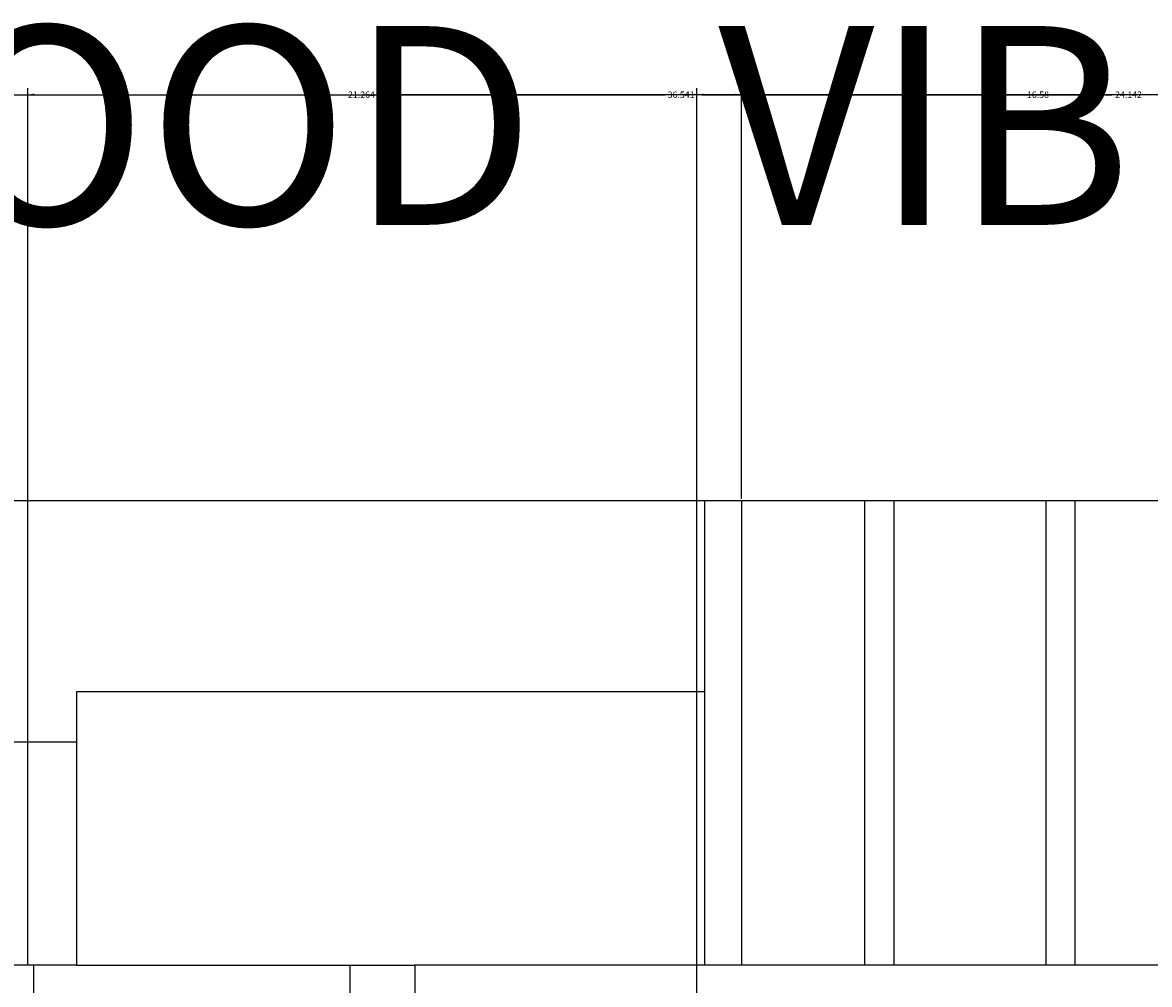
# Model space of a CAD drawing. Units: inches. Extents: x -117 to 121, y -77 to 40.
# Tile 28 of 45: x -23 to 9, y 14 to 40. Entities that reach past the tile are written whole.
import ezdxf

# ---------------------------------------------------------------- set-up
doc = ezdxf.new("R2010")
doc.units = ezdxf.units.IN
doc.header["$MEASUREMENT"] = 0
for name, color, linetype, lineweight in [('A-ANNO-DIMS', 2, 'Continuous', 18), ('A-ANNO-TEXT', 7, 'Continuous', 25), ('A-ELEV', 7, 'Continuous', 25)]:
    doc.layers.add(name, color=color, linetype=linetype, lineweight=lineweight)
doc.styles.get("Standard").update_dxf_attribs({"font": 'arial.ttf'})
doc.dimstyles.get("Standard").update_dxf_attribs({"dimtxt": 0.18, "dimasz": 0.18, "dimexe": 0.18, "dimexo": 0.0625, "dimgap": 0.09, "dimtad": 0, "dimtih": 1, "dimtoh": 1, "dimdec": 4, "dimzin": 0, "dimdsep": 46, "dimtxsty": 'Standard', "dimcen": 0.09, "dimadec": 0, "dimazin": 0, "dimtfac": 1, "dimtdec": 4, "dimtofl": 0, "dimtmove": 0, "dimatfit": 3, "dimfxl": 1, "dimtolj": 1, "dimtzin": 0, "dimarcsym": 0})

# ---------------------------------------------------------------- blocks, each defined once
blk = doc.blocks.new('*D10')
at = {"layer": 'A-ANNO-DIMS', "color": 0, "lineweight": -2, "transparency": 16777216}
for p, q in [((-2.6, 27.126), (-2.6, 38.61)), ((13.978, 27.126), (13.978, 38.61)), ((-2.42, 38.43), (5.304, 38.43)), ((13.798, 38.43), (6.075, 38.43))]:
    blk.add_line(p, q, dxfattribs=at)
at = {"layer": 'A-ANNO-DIMS', "color": 0, "transparency": 16777216}
for points in [[(-2.42, 38.46), (-2.42, 38.4), (-2.6, 38.43)], [(13.798, 38.46), (13.798, 38.4), (13.978, 38.43)]]:
    blk.add_solid(points, dxfattribs=at)
at = {"layer": 'Defpoints', "color": 0, "transparency": 16777216}
for p in [(13.978, 38.43), (-2.6, 27.063), (13.978, 27.063)]:
    blk.add_point(p, dxfattribs=at)
at = {"layer": 'A-ANNO-DIMS', "color": 0, "transparency": 16777216, "insert": (5.689, 38.43), "char_height": 0.18, "attachment_point": 5}
blk.add_mtext('\\A1;16.58', dxfattribs=at)
blk = doc.blocks.new('*D13')
at = {"layer": 'A-ANNO-DIMS', "color": 0, "lineweight": -2, "transparency": 16777216}
for p, q in [((-2.663, 27.063), (-117.024, 27.063)), ((-116.844, 26.883), (-116.844, -16.974)), ((-116.844, -61.196), (-116.844, -17.338)), ((-106.096, -61.376), (-117.024, -61.376))]:
    blk.add_line(p, q, dxfattribs=at)
at = {"layer": 'A-ANNO-DIMS', "color": 0, "transparency": 16777216}
for points in [[(-116.874, 26.883), (-116.814, 26.883), (-116.844, 27.063)], [(-116.874, -61.196), (-116.814, -61.196), (-116.844, -61.376)]]:
    blk.add_solid(points, dxfattribs=at)
at = {"layer": 'Defpoints', "color": 0, "transparency": 16777216}
for p in [(-2.6, 27.063), (-116.844, -61.376), (-106.034, -61.376)]:
    blk.add_point(p, dxfattribs=at)
at = {"layer": 'A-ANNO-DIMS', "color": 0, "transparency": 16777216, "insert": (-116.844, -17.156), "char_height": 0.18, "attachment_point": 5}
blk.add_mtext('\\A1;88.44', dxfattribs=at)
blk = doc.blocks.new('*D22')
at = {"layer": 'A-ANNO-DIMS', "color": 0, "lineweight": -2, "transparency": 16777216}
for p, q in [((-23.864, 8.087), (-23.864, 38.61)), ((-2.6, 27.126), (-2.6, 38.61)), ((-23.684, 38.43), (-13.697, 38.43)), ((-2.78, 38.43), (-12.767, 38.43))]:
    blk.add_line(p, q, dxfattribs=at)
at = {"layer": 'A-ANNO-DIMS', "color": 0, "transparency": 16777216}
for points in [[(-23.684, 38.46), (-23.684, 38.4), (-23.864, 38.43)], [(-2.78, 38.46), (-2.78, 38.4), (-2.6, 38.43)]]:
    blk.add_solid(points, dxfattribs=at)
at = {"layer": 'Defpoints', "color": 0, "transparency": 16777216}
for p in [(-2.6, 38.43), (-2.6, 27.063), (-23.864, 8.025)]:
    blk.add_point(p, dxfattribs=at)
at = {"layer": 'A-ANNO-DIMS', "color": 0, "transparency": 16777216, "insert": (-13.232, 38.43), "char_height": 0.18, "attachment_point": 5}
blk.add_mtext('\\A1;21.264', dxfattribs=at)
blk = doc.blocks.new('*D32')
at = {"layer": 'A-ANNO-DIMS', "color": 0, "lineweight": -2, "transparency": 16777216}
for p, q in [((-3.85, -45.55), (-3.85, 38.61)), ((20.293, -45.55), (20.293, 38.61)), ((-3.67, 38.43), (7.757, 38.43)), ((20.113, 38.43), (8.686, 38.43))]:
    blk.add_line(p, q, dxfattribs=at)
at = {"layer": 'A-ANNO-DIMS', "color": 0, "transparency": 16777216}
for points in [[(-3.67, 38.46), (-3.67, 38.4), (-3.85, 38.43)], [(20.113, 38.46), (20.113, 38.4), (20.293, 38.43)]]:
    blk.add_solid(points, dxfattribs=at)
at = {"layer": 'Defpoints', "color": 0, "transparency": 16777216}
for p in [(20.293, 38.43), (-3.85, -45.613), (20.293, -45.613)]:
    blk.add_point(p, dxfattribs=at)
at = {"layer": 'A-ANNO-DIMS', "color": 0, "transparency": 16777216, "insert": (8.222, 38.43), "char_height": 0.18, "attachment_point": 5}
blk.add_mtext('\\A1;24.142', dxfattribs=at)
blk = doc.blocks.new('*D51')
at = {"layer": 'A-ANNO-DIMS', "color": 0, "lineweight": -2, "transparency": 16777216}
for p, q in [((-22.563, 14.079), (-22.563, 38.61)), ((13.978, 14.136), (13.978, 38.61)), ((-22.383, 38.43), (-4.738, 38.43)), ((13.798, 38.43), (-3.846, 38.43))]:
    blk.add_line(p, q, dxfattribs=at)
at = {"layer": 'A-ANNO-DIMS', "color": 0, "transparency": 16777216}
for points in [[(-22.383, 38.46), (-22.383, 38.4), (-22.563, 38.43)], [(13.798, 38.46), (13.798, 38.4), (13.978, 38.43)]]:
    blk.add_solid(points, dxfattribs=at)
at = {"layer": 'Defpoints', "color": 0, "transparency": 16777216}
for p in [(13.978, 38.43), (-22.563, 14.016), (13.978, 14.074)]:
    blk.add_point(p, dxfattribs=at)
at = {"layer": 'A-ANNO-DIMS', "color": 0, "transparency": 16777216, "insert": (-4.292, 38.43), "char_height": 0.18, "attachment_point": 5}
blk.add_mtext('\\A1;36.541', dxfattribs=at)

msp = doc.modelspace()

# ---------------------------------------------------------------- linework, layer by layer
at = {"layer": 'A-ELEV'}
for p, q in [((13.9784, 27.0634), (-3.6347, 27.0634)), ((-3.6347, 27.0634), (-3.6347, 14.0735)), ((-2.6001, 27.0634), (-2.6001, 14.0735)), ((0.8395, 27.0634), (0.8395, 14.0735)), ((1.6541, 27.0634), (1.6541, 14.0735)), ((5.9083, 27.0634), (5.9083, 14.0735)), ((6.723, 27.0634), (6.723, 14.0735)), ((-21.1993, 21.7235), (-21.1993, 14.0735)), ((-3.6347, 21.7235), (-21.1993, 21.7235)), ((-21.1993, 20.3104), (-39.0355, 20.3104)), ((-21.1993, 14.0735), (-23.8637, 14.0735)), ((-22.4056, 14.0735), (-22.4056, -14.3771)), ((-21.1993, 14.0735), (-11.738, 14.0735)), ((-13.5598, 14.0735), (-13.5598, 2.5407)), ((13.9784, 14.0735), (-11.738, 14.0735)), ((-11.738, 14.0735), (-11.738, 2.5577))]:
    msp.add_line(p, q, dxfattribs=at)

# ---------------------------------------------------------------- texts
at = {"layer": 'A-ANNO-TEXT'}
msp.add_text('CONCEPTUAL    GOOD   VIBE   CAFE   DESIGN', height=5.56486, dxfattribs=at).set_placement((-85.726, 34.7863))

# ---------------------------------------------------------------- dimensions: what is measured, and where the dimension line sits
at = {"layer": 'A-ANNO-DIMS'}
for base, p1, p2, override, picture, middle in [((-2.6001, 38.4297), (-23.8637, 8.0246), (-2.6001, 27.0634), {"dimdec": 3, "dimlfac": 1, "dimrnd": 0, "dimzin": 0, "dimdsep": 46, "dimlunit": 2}, '*D22', (-13.2319, 38.4297)), ((13.9784, 38.4297), (-22.5628, 14.0161), (13.9784, 14.0735), {"dimdec": 3, "dimlfac": 1, "dimrnd": 0, "dimzin": 0, "dimdsep": 46, "dimlunit": 2}, '*D51', (-4.2922, 38.4297)), ((20.2929, 38.4297), (-3.8495, -45.6125), (20.2929, -45.6125), {"dimdec": 3, "dimlfac": 1, "dimrnd": 0, "dimzin": 0, "dimdsep": 46, "dimlunit": 2}, '*D32', (8.2217, 38.4297)), ((13.9784, 38.4297), (-2.6001, 27.0634), (13.9784, 27.0634), {"dimdec": 2, "dimlfac": 1, "dimrnd": 0, "dimzin": 0, "dimdsep": 46, "dimlunit": 2}, '*D10', (5.6892, 38.4297))]:
    dim = msp.add_linear_dim(base=base, p1=p1, p2=p2, dimstyle='Standard', override=override, dxfattribs=at)
    dim.commit()
    dim.dimension.update_dxf_attribs({"geometry": picture, "text_midpoint": middle})
dim = msp.add_linear_dim(base=(-116.8438, -61.3756), p1=(-2.6001, 27.0634), p2=(-106.0338, -61.3756), angle=90, dimstyle='Standard', override={"dimdec": 2, "dimlfac": 1, "dimrnd": 0, "dimzin": 0, "dimdsep": 46, "dimlunit": 2}, dxfattribs=at)
dim.commit()
dim.dimension.update_dxf_attribs({"geometry": '*D13', "text_midpoint": (-116.8438, -17.1561)})

doc.saveas('drawing.dxf')
